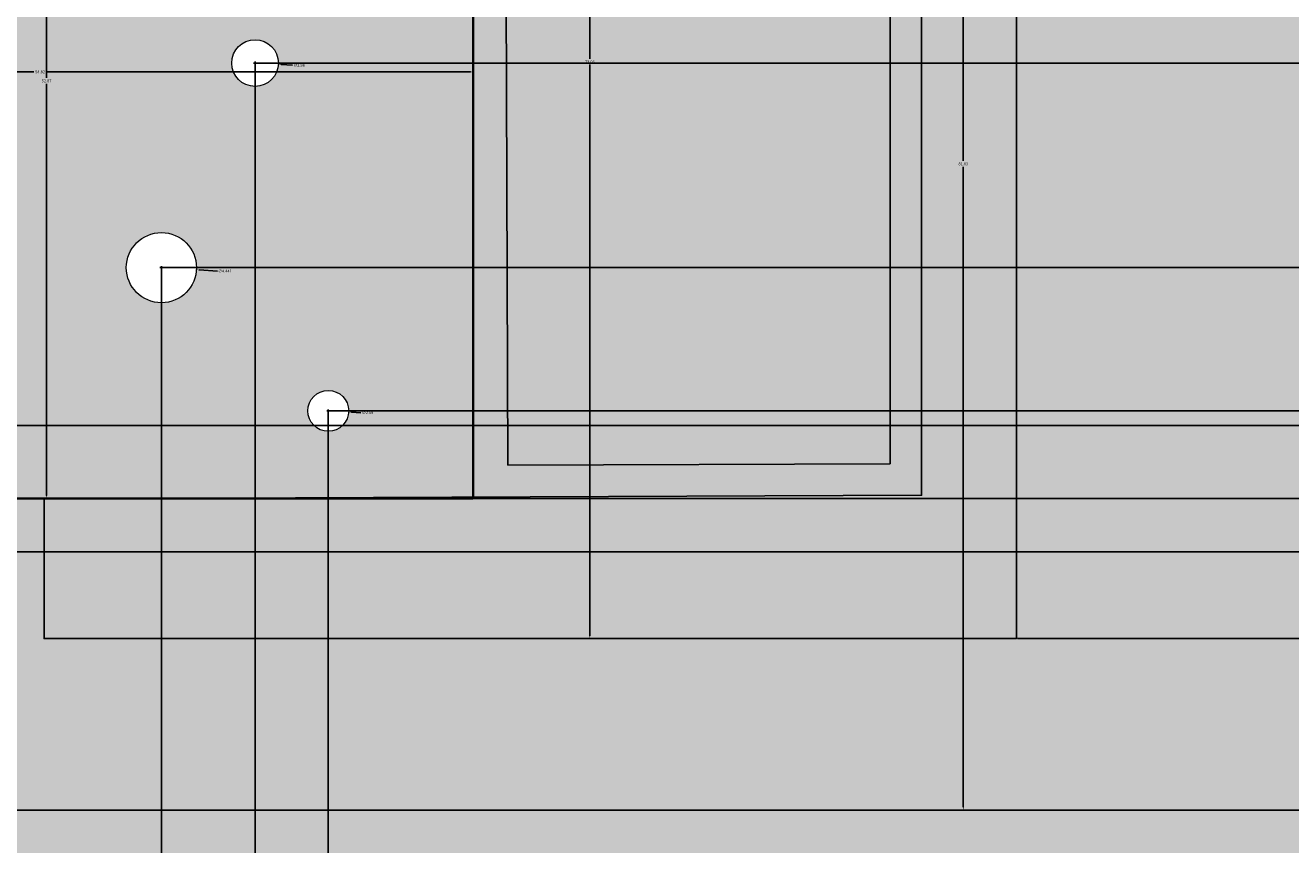
# Model space of a CAD drawing. Units: inches. Extents: x 73 to 607, y 92 to 651.
# Tile 4 of 18: x 368 to 448, y 173 to 224. Entities that reach past the tile are written whole.
import ezdxf

# ---------------------------------------------------------------- set-up
doc = ezdxf.new("R2010")
doc.units = ezdxf.units.IN
doc.header["$MEASUREMENT"] = 0
for name, color, linetype, lineweight in [('A-ANNO-DIMS', 2, 'Continuous', 18), ('A-ELEV', 7, 'Continuous', 35), ('A-ELEV-PANL', 7, 'Continuous', 18), ('A-ELEV-PATT-BKGD', 252, 'Continuous', 13), ('A-ELEV-PATT-FRAM', 38, 'Continuous', 13), ('A-ELEV-PATT-SHAD', 8, 'Continuous', 13), ('A-ELEV-PATT-WALL', 254, 'Continuous', 13), ('A-ELEV-PATT-WOOD', 32, 'Continuous', 13), ('A-GLAZ', 4, 'Continuous', 25), ('A-GLAZ-PATT', 7, 'Continuous', 13)]:
    doc.layers.add(name, color=color, linetype=linetype, lineweight=lineweight)
doc.styles.get("Standard").update_dxf_attribs({"font": 'arial.ttf'})
doc.dimstyles.get("Standard").update_dxf_attribs({"dimtxt": 0.18, "dimasz": 0.18, "dimexe": 0.18, "dimexo": 0.0625, "dimgap": 0.09, "dimtad": 0, "dimtih": 1, "dimtoh": 1, "dimdec": 4, "dimzin": 0, "dimdsep": 46, "dimtxsty": 'Standard', "dimcen": 0.09, "dimadec": 0, "dimazin": 0, "dimtfac": 1, "dimtdec": 4, "dimtofl": 0, "dimtmove": 0, "dimatfit": 3, "dimfxl": 1, "dimtolj": 1, "dimtzin": 0, "dimarcsym": 0})

# ---------------------------------------------------------------- blocks, each defined once
blk = doc.blocks.new('*D16')
at = {"layer": 'A-ANNO-DIMS', "color": 0, "lineweight": -2, "transparency": 16777216}
for p, q in [((431.133, 185.662), (607.278, 185.662)), ((607.098, 185.482), (607.098, 180.414)), ((607.098, 174.982), (607.098, 180.05)), ((454.767, 174.802), (607.278, 174.802))]:
    blk.add_line(p, q, dxfattribs=at)
at = {"layer": 'A-ANNO-DIMS', "color": 0, "transparency": 16777216}
for points in [[(607.068, 185.482), (607.128, 185.482), (607.098, 185.662)], [(607.068, 174.982), (607.128, 174.982), (607.098, 174.802)]]:
    blk.add_solid(points, dxfattribs=at)
at = {"layer": 'Defpoints', "color": 0, "transparency": 16777216}
for p in [(431.07, 185.662), (607.098, 185.662), (454.705, 174.802)]:
    blk.add_point(p, dxfattribs=at)
at = {"layer": 'A-ANNO-DIMS', "color": 0, "transparency": 16777216, "insert": (607.098, 180.232), "char_height": 0.18, "attachment_point": 5}
blk.add_mtext('\\A1;10.86', dxfattribs=at)
blk = doc.blocks.new('*D17')
at = {"layer": 'A-ANNO-DIMS', "color": 0, "lineweight": -2, "transparency": 16777216}
for p, q in [((580.161, 262.302), (607.278, 262.302)), ((607.098, 262.122), (607.098, 224.164)), ((607.098, 185.842), (607.098, 223.8)), ((431.133, 185.662), (607.278, 185.662))]:
    blk.add_line(p, q, dxfattribs=at)
at = {"layer": 'A-ANNO-DIMS', "color": 0, "transparency": 16777216}
for points in [[(607.068, 262.122), (607.128, 262.122), (607.098, 262.302)], [(607.068, 185.842), (607.128, 185.842), (607.098, 185.662)]]:
    blk.add_solid(points, dxfattribs=at)
at = {"layer": 'Defpoints', "color": 0, "transparency": 16777216}
for p in [(580.098, 262.302), (607.098, 262.302), (431.07, 185.662)]:
    blk.add_point(p, dxfattribs=at)
at = {"layer": 'A-ANNO-DIMS', "color": 0, "transparency": 16777216, "insert": (607.098, 223.982), "char_height": 0.18, "attachment_point": 5}
blk.add_mtext('\\A1;76.64', dxfattribs=at)
blk = doc.blocks.new('*D35')
at = {"layer": 'A-ANNO-DIMS', "color": 0, "lineweight": -2, "transparency": 16777216}
for p, q in [((341.869, 194.608), (341.873, 221.725)), ((342.053, 221.545), (368.892, 221.541)), ((396.516, 221.537), (369.677, 221.541)), ((396.692, 194.599), (396.696, 221.717))]:
    blk.add_line(p, q, dxfattribs=at)
at = {"layer": 'A-ANNO-DIMS', "color": 0, "transparency": 16777216}
for points in [[(342.053, 221.575), (342.053, 221.515), (341.873, 221.545)], [(396.516, 221.567), (396.516, 221.507), (396.696, 221.537)]]:
    blk.add_solid(points, dxfattribs=at)
at = {"layer": 'Defpoints', "color": 0, "transparency": 16777216}
for p in [(396.696, 221.537), (341.869, 194.545), (396.692, 194.537)]:
    blk.add_point(p, dxfattribs=at)
at = {"layer": 'A-ANNO-DIMS', "color": 0, "transparency": 16777216, "insert": (369.285, 221.541), "char_height": 0.18, "attachment_point": 5}
blk.add_mtext('\\A1;54.82', dxfattribs=at)
blk = doc.blocks.new('*D36')
at = {"layer": 'A-ANNO-DIMS', "color": 0, "lineweight": -2, "transparency": 16777216}
for p, q in [((396.63, 247.405), (369.512, 247.405)), ((369.692, 247.225), (369.692, 221.153)), ((369.692, 194.717), (369.692, 220.789)), ((396.63, 194.537), (369.512, 194.537))]:
    blk.add_line(p, q, dxfattribs=at)
at = {"layer": 'A-ANNO-DIMS', "color": 0, "transparency": 16777216}
for points in [[(369.662, 247.225), (369.722, 247.225), (369.692, 247.405)], [(369.662, 194.717), (369.722, 194.717), (369.692, 194.537)]]:
    blk.add_solid(points, dxfattribs=at)
at = {"layer": 'Defpoints', "color": 0, "transparency": 16777216}
for p in [(369.692, 247.405), (396.692, 247.405), (396.692, 194.537)]:
    blk.add_point(p, dxfattribs=at)
at = {"layer": 'A-ANNO-DIMS', "color": 0, "transparency": 16777216, "insert": (369.692, 220.971), "char_height": 0.18, "attachment_point": 5}
blk.add_mtext('\\A1;52.87', dxfattribs=at)
blk = doc.blocks.new('*D38')
at = {"layer": 'A-ANNO-DIMS', "color": 0, "lineweight": -2, "transparency": 16777216}
for p, q in [((431.008, 258.691), (403.89, 258.691)), ((404.07, 258.511), (404.07, 222.359)), ((404.07, 185.842), (404.07, 221.995)), ((431.008, 185.662), (403.89, 185.662))]:
    blk.add_line(p, q, dxfattribs=at)
at = {"layer": 'A-ANNO-DIMS', "color": 0, "transparency": 16777216}
for points in [[(404.04, 258.511), (404.1, 258.511), (404.07, 258.691)], [(404.04, 185.842), (404.1, 185.842), (404.07, 185.662)]]:
    blk.add_solid(points, dxfattribs=at)
at = {"layer": 'Defpoints', "color": 0, "transparency": 16777216}
for p in [(404.07, 258.691), (431.07, 258.691), (431.07, 185.662)]:
    blk.add_point(p, dxfattribs=at)
at = {"layer": 'A-ANNO-DIMS', "color": 0, "transparency": 16777216, "insert": (404.07, 222.177), "char_height": 0.18, "attachment_point": 5}
blk.add_mtext('\\A1;73.03', dxfattribs=at)
blk = doc.blocks.new('*D40')
at = {"layer": 'A-ANNO-DIMS', "color": 0, "lineweight": -2, "transparency": 16777216}
for p, q in [((454.642, 256.632), (427.525, 256.632)), ((427.705, 256.452), (427.705, 215.899)), ((427.705, 174.982), (427.705, 215.535)), ((454.642, 174.802), (427.525, 174.802))]:
    blk.add_line(p, q, dxfattribs=at)
at = {"layer": 'A-ANNO-DIMS', "color": 0, "transparency": 16777216}
for points in [[(427.675, 256.452), (427.735, 256.452), (427.705, 256.632)], [(427.675, 174.982), (427.735, 174.982), (427.705, 174.802)]]:
    blk.add_solid(points, dxfattribs=at)
at = {"layer": 'Defpoints', "color": 0, "transparency": 16777216}
for p in [(427.705, 256.632), (454.705, 256.632), (454.705, 174.802)]:
    blk.add_point(p, dxfattribs=at)
at = {"layer": 'A-ANNO-DIMS', "color": 0, "transparency": 16777216, "insert": (427.705, 215.717), "char_height": 0.18, "attachment_point": 5}
blk.add_mtext('\\A1;81.83', dxfattribs=at)
blk = doc.blocks.new('*D88')
at = {"layer": 'A-ANNO-DIMS', "color": 0, "lineweight": -2, "transparency": 16777216}
for p, q in [((376.96, 209.081), (376.96, 116.024)), ((363.256, 199.089), (363.256, 116.024)), ((363.436, 116.204), (369.654, 116.204)), ((376.78, 116.204), (370.563, 116.204))]:
    blk.add_line(p, q, dxfattribs=at)
at = {"layer": 'A-ANNO-DIMS', "color": 0, "transparency": 16777216}
for points in [[(363.436, 116.234), (363.436, 116.174), (363.256, 116.204)], [(376.78, 116.234), (376.78, 116.174), (376.96, 116.204)]]:
    blk.add_solid(points, dxfattribs=at)
at = {"layer": 'Defpoints', "color": 0, "transparency": 16777216}
for p in [(376.96, 209.143), (363.256, 199.151), (376.96, 116.204)]:
    blk.add_point(p, dxfattribs=at)
at = {"layer": 'A-ANNO-DIMS', "color": 0, "transparency": 16777216, "insert": (370.108, 116.204), "char_height": 0.18, "attachment_point": 5}
blk.add_mtext('\\A1;13.704', dxfattribs=at)
blk = doc.blocks.new('*D89')
at = {"layer": 'A-ANNO-DIMS', "color": 0, "lineweight": -2, "transparency": 16777216}
for p, q in [((382.886, 222.034), (382.886, 116.024)), ((376.96, 209.081), (376.96, 116.024)), ((377.14, 116.204), (379.53, 116.204)), ((382.706, 116.204), (380.317, 116.204))]:
    blk.add_line(p, q, dxfattribs=at)
at = {"layer": 'A-ANNO-DIMS', "color": 0, "transparency": 16777216}
for points in [[(377.14, 116.234), (377.14, 116.174), (376.96, 116.204)], [(382.706, 116.234), (382.706, 116.174), (382.886, 116.204)]]:
    blk.add_solid(points, dxfattribs=at)
at = {"layer": 'Defpoints', "color": 0, "transparency": 16777216}
for p in [(382.886, 222.096), (376.96, 209.143), (382.886, 116.204)]:
    blk.add_point(p, dxfattribs=at)
at = {"layer": 'A-ANNO-DIMS', "color": 0, "transparency": 16777216, "insert": (379.923, 116.204), "char_height": 0.18, "attachment_point": 5}
blk.add_mtext('\\A1;5.926', dxfattribs=at)
blk = doc.blocks.new('*D90')
at = {"layer": 'A-ANNO-DIMS', "color": 0, "lineweight": -2, "transparency": 16777216}
for p, q in [((382.886, 222.034), (382.886, 116.024)), ((387.516, 200.014), (387.516, 116.024)), ((383.066, 116.204), (384.874, 116.204)), ((387.336, 116.204), (385.529, 116.204))]:
    blk.add_line(p, q, dxfattribs=at)
at = {"layer": 'A-ANNO-DIMS', "color": 0, "transparency": 16777216}
for points in [[(383.066, 116.234), (383.066, 116.174), (382.886, 116.204)], [(387.336, 116.234), (387.336, 116.174), (387.516, 116.204)]]:
    blk.add_solid(points, dxfattribs=at)
at = {"layer": 'Defpoints', "color": 0, "transparency": 16777216}
for p in [(382.886, 222.096), (387.516, 200.076), (387.516, 116.204)]:
    blk.add_point(p, dxfattribs=at)
at = {"layer": 'A-ANNO-DIMS', "color": 0, "transparency": 16777216, "insert": (385.201, 116.204), "char_height": 0.18, "attachment_point": 5}
blk.add_mtext('\\A1;4.63', dxfattribs=at)
blk = doc.blocks.new('*D94')
at = {"layer": 'A-ANNO-DIMS', "color": 0, "lineweight": -2, "transparency": 16777216}
for p, q in [((377.023, 209.143), (607.278, 209.143)), ((607.098, 208.963), (607.098, 204.329)), ((607.098, 199.331), (607.098, 203.965)), ((363.319, 199.151), (607.278, 199.151))]:
    blk.add_line(p, q, dxfattribs=at)
at = {"layer": 'A-ANNO-DIMS', "color": 0, "transparency": 16777216}
for points in [[(607.068, 208.963), (607.128, 208.963), (607.098, 209.143)], [(607.068, 199.331), (607.128, 199.331), (607.098, 199.151)]]:
    blk.add_solid(points, dxfattribs=at)
at = {"layer": 'Defpoints', "color": 0, "transparency": 16777216}
for p in [(376.96, 209.143), (363.256, 199.151), (607.098, 199.151)]:
    blk.add_point(p, dxfattribs=at)
at = {"layer": 'A-ANNO-DIMS', "color": 0, "transparency": 16777216, "insert": (607.098, 204.147), "char_height": 0.18, "attachment_point": 5}
blk.add_mtext('\\A1;9.992', dxfattribs=at)
blk = doc.blocks.new('*D95')
at = {"layer": 'A-ANNO-DIMS', "color": 0, "lineweight": -2, "transparency": 16777216}
for p, q in [((363.874, 225.982), (607.278, 225.982)), ((607.098, 225.802), (607.098, 212.749)), ((607.098, 199.331), (607.098, 212.385)), ((363.319, 199.151), (607.278, 199.151))]:
    blk.add_line(p, q, dxfattribs=at)
at = {"layer": 'A-ANNO-DIMS', "color": 0, "transparency": 16777216}
for points in [[(607.068, 225.802), (607.128, 225.802), (607.098, 225.982)], [(607.068, 199.331), (607.128, 199.331), (607.098, 199.151)]]:
    blk.add_solid(points, dxfattribs=at)
at = {"layer": 'Defpoints', "color": 0, "transparency": 16777216}
for p in [(363.812, 225.982), (607.098, 225.982), (363.256, 199.151)]:
    blk.add_point(p, dxfattribs=at)
at = {"layer": 'A-ANNO-DIMS', "color": 0, "transparency": 16777216, "insert": (607.098, 212.567), "char_height": 0.18, "attachment_point": 5}
blk.add_mtext('\\A1;26.83', dxfattribs=at)
blk = doc.blocks.new('*D97')
at = {"layer": 'A-ANNO-DIMS', "color": 0, "lineweight": -2, "transparency": 16777216}
for p, q in [((387.579, 200.076), (607.278, 200.076)), ((607.098, 199.896), (607.098, 197.488)), ((607.098, 194.717), (607.098, 197.125)), ((396.755, 194.537), (607.278, 194.537))]:
    blk.add_line(p, q, dxfattribs=at)
at = {"layer": 'A-ANNO-DIMS', "color": 0, "transparency": 16777216}
for points in [[(607.068, 199.896), (607.128, 199.896), (607.098, 200.076)], [(607.068, 194.717), (607.128, 194.717), (607.098, 194.537)]]:
    blk.add_solid(points, dxfattribs=at)
at = {"layer": 'Defpoints', "color": 0, "transparency": 16777216}
for p in [(387.516, 200.076), (607.098, 200.076), (396.692, 194.537)]:
    blk.add_point(p, dxfattribs=at)
at = {"layer": 'A-ANNO-DIMS', "color": 0, "transparency": 16777216, "insert": (607.098, 197.306), "char_height": 0.18, "attachment_point": 5}
blk.add_mtext('\\A1;5.54', dxfattribs=at)
blk = doc.blocks.new('*D98')
at = {"layer": 'A-ANNO-DIMS', "color": 0, "lineweight": -2, "transparency": 16777216}
for p, q in [((377.023, 209.143), (607.278, 209.143)), ((607.098, 208.963), (607.098, 204.792)), ((607.098, 200.256), (607.098, 204.428)), ((387.579, 200.076), (607.278, 200.076))]:
    blk.add_line(p, q, dxfattribs=at)
at = {"layer": 'A-ANNO-DIMS', "color": 0, "transparency": 16777216}
for points in [[(607.068, 208.963), (607.128, 208.963), (607.098, 209.143)], [(607.068, 200.256), (607.128, 200.256), (607.098, 200.076)]]:
    blk.add_solid(points, dxfattribs=at)
at = {"layer": 'Defpoints', "color": 0, "transparency": 16777216}
for p in [(376.96, 209.143), (607.098, 209.143), (387.516, 200.076)]:
    blk.add_point(p, dxfattribs=at)
at = {"layer": 'A-ANNO-DIMS', "color": 0, "transparency": 16777216, "insert": (607.098, 204.61), "char_height": 0.18, "attachment_point": 5}
blk.add_mtext('\\A1;9.067', dxfattribs=at)
blk = doc.blocks.new('*D99')
at = {"layer": 'A-ANNO-DIMS', "color": 0, "lineweight": -2, "transparency": 16777216}
for p, q in [((373.319, 231.348), (607.278, 231.348)), ((607.098, 231.168), (607.098, 220.428)), ((607.098, 209.323), (607.098, 220.064)), ((377.023, 209.143), (607.278, 209.143))]:
    blk.add_line(p, q, dxfattribs=at)
at = {"layer": 'A-ANNO-DIMS', "color": 0, "transparency": 16777216}
for points in [[(607.068, 231.168), (607.128, 231.168), (607.098, 231.348)], [(607.068, 209.323), (607.128, 209.323), (607.098, 209.143)]]:
    blk.add_solid(points, dxfattribs=at)
at = {"layer": 'Defpoints', "color": 0, "transparency": 16777216}
for p in [(373.257, 231.348), (607.098, 231.348), (376.96, 209.143)]:
    blk.add_point(p, dxfattribs=at)
at = {"layer": 'A-ANNO-DIMS', "color": 0, "transparency": 16777216, "insert": (607.098, 220.246), "char_height": 0.18, "attachment_point": 5}
blk.add_mtext('\\A1;22.205', dxfattribs=at)
blk = doc.blocks.new('*D100')
at = {"layer": 'A-ANNO-DIMS', "color": 0, "lineweight": -2, "transparency": 16777216}
for p, q in [((382.949, 222.096), (607.278, 222.096)), ((607.098, 221.916), (607.098, 211.268)), ((607.098, 200.256), (607.098, 210.904)), ((387.579, 200.076), (607.278, 200.076))]:
    blk.add_line(p, q, dxfattribs=at)
at = {"layer": 'A-ANNO-DIMS', "color": 0, "transparency": 16777216}
for points in [[(607.068, 221.916), (607.128, 221.916), (607.098, 222.096)], [(607.068, 200.256), (607.128, 200.256), (607.098, 200.076)]]:
    blk.add_solid(points, dxfattribs=at)
at = {"layer": 'Defpoints', "color": 0, "transparency": 16777216}
for p in [(382.886, 222.096), (607.098, 222.096), (387.516, 200.076)]:
    blk.add_point(p, dxfattribs=at)
at = {"layer": 'A-ANNO-DIMS', "color": 0, "transparency": 16777216, "insert": (607.098, 211.086), "char_height": 0.18, "attachment_point": 5}
blk.add_mtext('\\A1;22.02', dxfattribs=at)
blk = doc.blocks.new('*D101')
at = {"layer": 'A-ANNO-DIMS', "color": 0, "lineweight": -2, "transparency": 16777216}
for p, q in [((382.393, 240.97), (607.278, 240.97)), ((607.098, 240.79), (607.098, 231.715)), ((607.098, 222.276), (607.098, 231.351)), ((382.949, 222.096), (607.278, 222.096))]:
    blk.add_line(p, q, dxfattribs=at)
at = {"layer": 'A-ANNO-DIMS', "color": 0, "transparency": 16777216}
for points in [[(607.068, 240.79), (607.128, 240.79), (607.098, 240.97)], [(607.068, 222.276), (607.128, 222.276), (607.098, 222.096)]]:
    blk.add_solid(points, dxfattribs=at)
at = {"layer": 'Defpoints', "color": 0, "transparency": 16777216}
for p in [(382.331, 240.97), (607.098, 240.97), (382.886, 222.096)]:
    blk.add_point(p, dxfattribs=at)
at = {"layer": 'A-ANNO-DIMS', "color": 0, "transparency": 16777216, "insert": (607.098, 231.533), "char_height": 0.18, "attachment_point": 5}
blk.add_mtext('\\A1;18.874', dxfattribs=at)
blk = doc.blocks.new('*D119')
at = {"layer": 'A-ANNO-DIMS', "color": 0, "lineweight": -2, "transparency": 16777216}
for p, q in [((469.817, 191.142), (72.918, 191.142)), ((73.098, 190.962), (73.098, 183.154)), ((73.098, 174.982), (73.098, 182.79)), ((454.642, 174.802), (72.918, 174.802))]:
    blk.add_line(p, q, dxfattribs=at)
at = {"layer": 'A-ANNO-DIMS', "color": 0, "transparency": 16777216}
for points in [[(73.068, 190.962), (73.128, 190.962), (73.098, 191.142)], [(73.068, 174.982), (73.128, 174.982), (73.098, 174.802)]]:
    blk.add_solid(points, dxfattribs=at)
at = {"layer": 'Defpoints', "color": 0, "transparency": 16777216}
for p in [(73.098, 191.142), (469.879, 191.142), (454.705, 174.802)]:
    blk.add_point(p, dxfattribs=at)
at = {"layer": 'A-ANNO-DIMS', "color": 0, "transparency": 16777216, "insert": (73.098, 182.972), "char_height": 0.18, "attachment_point": 5}
blk.add_mtext('\\A1;16.34', dxfattribs=at)
blk = doc.blocks.new('*D149')
at = {"layer": 'A-ANNO-DIMS', "color": 0, "lineweight": -2, "transparency": 16777216}
for p, q in [((382.796, 222.096), (382.976, 222.096)), ((382.886, 222.006), (382.886, 222.186)), ((385.251, 221.954), (384.544, 221.997))]:
    blk.add_line(p, q, dxfattribs=at)
at = {"layer": 'A-ANNO-DIMS', "color": 0, "transparency": 16777216}
blk.add_solid([(384.546, 222.027), (384.542, 221.967), (384.364, 222.008)], dxfattribs=at)
at = {"layer": 'Defpoints', "color": 0, "transparency": 16777216}
for p in [(381.409, 222.185), (384.364, 222.008)]:
    blk.add_point(p, dxfattribs=at)
at = {"layer": 'A-ANNO-DIMS', "color": 0, "transparency": 16777216, "insert": (385.672, 221.954), "char_height": 0.18, "attachment_point": 5}
blk.add_mtext('\\A1;∅2.96', dxfattribs=at)
blk = doc.blocks.new('*D151')
at = {"layer": 'A-ANNO-DIMS', "color": 0, "lineweight": -2, "transparency": 16777216}
for p, q in [((376.87, 209.143), (377.05, 209.143)), ((376.96, 209.053), (376.96, 209.233)), ((380.507, 208.928), (379.356, 208.998))]:
    blk.add_line(p, q, dxfattribs=at)
at = {"layer": 'A-ANNO-DIMS', "color": 0, "transparency": 16777216}
blk.add_solid([(379.358, 209.028), (379.355, 208.968), (379.177, 209.009)], dxfattribs=at)
at = {"layer": 'Defpoints', "color": 0, "transparency": 16777216}
for p in [(374.744, 209.278), (379.177, 209.009)]:
    blk.add_point(p, dxfattribs=at)
at = {"layer": 'A-ANNO-DIMS', "color": 0, "transparency": 16777216, "insert": (380.981, 208.928), "char_height": 0.18, "attachment_point": 5}
blk.add_mtext('\\A1;∅4.441', dxfattribs=at)
blk = doc.blocks.new('*D153')
at = {"layer": 'A-ANNO-DIMS', "color": 0, "lineweight": -2, "transparency": 16777216}
for p, q in [((387.426, 200.076), (387.606, 200.076)), ((387.516, 199.986), (387.516, 200.166)), ((389.585, 199.961), (388.989, 199.994))]:
    blk.add_line(p, q, dxfattribs=at)
at = {"layer": 'A-ANNO-DIMS', "color": 0, "transparency": 16777216}
blk.add_solid([(388.991, 200.024), (388.987, 199.965), (388.809, 200.004)], dxfattribs=at)
at = {"layer": 'Defpoints', "color": 0, "transparency": 16777216}
for p in [(386.223, 200.148), (388.809, 200.004)]:
    blk.add_point(p, dxfattribs=at)
at = {"layer": 'A-ANNO-DIMS', "color": 0, "transparency": 16777216, "insert": (390.007, 199.961), "char_height": 0.18, "attachment_point": 5}
blk.add_mtext('\\A1;∅2.59', dxfattribs=at)

msp = doc.modelspace()

# ---------------------------------------------------------------- hatches: boundary and pattern name
at = {"layer": 'A-ELEV-PATT-BKGD'}
h = msp.add_hatch(color=256, dxfattribs=at)
h.dxf.hatch_style = 1
h.paths.add_polyline_path([(321.3008, 479.2042), (312.3008, 479.2042), (312.3008, 478.7576), (312.3008, 412.636), (321.3008, 412.636)])
h.paths.add_polyline_path([(312.3008, 504.7576), (256.4726, 504.7576), (256.4726, 503.4576), (312.3008, 503.4576)], flags=17)
h.paths.add_polyline_path([(321.3008, 543.1576), (321.3008, 552.1576), (320.3257, 552.1576), (312.3008, 552.1576), (256.4726, 552.1576), (256.4726, 543.1576), (312.3008, 543.1576), (312.3008, 479.2042), (321.3008, 479.2042)])
h.paths.add_polyline_path([(451.5214, 412.636), (256.4726, 412.636), (256.4726, 403.636), (442.5214, 403.636), (442.5214, 320.2042), (206.1343, 320.2042), (206.1343, 320.9135), (206.1343, 403.636), (256.4726, 403.636), (256.4726, 412.636), (201.6343, 412.636), (201.6343, 320.9135), (201.6343, 320.2042), (201.6343, 311.2042), (256.4726, 311.2042), (451.5214, 311.2042)])
h.paths.add_polyline_path([(431.07, 258.6914), (369.5339, 258.6914), (369.5339, 247.4054), (396.692, 247.4054), (425.07, 247.4054), (425.07, 194.7312), (396.692, 194.6197), (396.692, 194.5366), (369.5339, 194.5366), (369.5339, 185.6619), (431.07, 185.6619)])
h.paths.add_polyline_path([(580.0983, 262.3024), (451.5214, 262.3024), (451.5214, 143.2042), (580.0983, 143.2042)])
h.paths.add_polyline_path([(454.7049, 174.802), (454.7049, 256.6321), (577.9249, 256.6321), (577.9249, 174.802)], flags=16)
h.paths.add_polyline_path([(465.9716, 191.1416, -1), (473.7874, 191.1416, -1)], flags=0)
h.paths.add_polyline_path([(490.5373, 181.6586, -1), (494.9999, 181.6586, -1)], flags=0)
h.paths.add_polyline_path([(476.2996, 209.8287, -1), (500.5844, 209.8287, -1)], flags=0)
h.paths.add_polyline_path([(505.3326, 194.7675, -1), (512.5843, 194.7675, -1)], flags=0)
h.paths.add_polyline_path([(520.9613, 186.679, -1), (526.544, 186.679, -1)], flags=0)
h.paths.add_polyline_path([(466.8103, 225.7267, -1), (470.1573, 225.7267, -1)], flags=0)
h.paths.add_polyline_path([(527.1059, 203.6926, -1), (536.0311, 203.6926, -1)], flags=0)
h.paths.add_polyline_path([(504.775, 232.6995, -1), (513.7002, 232.6995, -1)], flags=0)
h.paths.add_polyline_path([(546.9241, 183.611, -1), (554.7336, 183.611, -1)], flags=0)
h.paths.add_polyline_path([(459.5544, 243.856, -1), (466.8061, 243.856, -1)], flags=0)
h.paths.add_polyline_path([(476.3045, 246.924, -1), (488.5767, 246.924, -1)], flags=0)
h.paths.add_polyline_path([(529.9044, 226.8424, -1), (556.68, 226.8424, -1)], flags=0)
h.paths.add_polyline_path([(554.1814, 203.9716, -1), (561.4331, 203.9716, -1)], flags=0)
h.paths.add_polyline_path([(567.8561, 193.3729, -1), (570.6475, 193.3729, -1)], flags=0)
h.paths.add_polyline_path([(522.3584, 250.271, -1), (525.7053, 250.271, -1)], flags=0)
h.paths.add_polyline_path([(561.9965, 245.2506, -1), (567.5748, 245.2506, -1)], flags=0)
h.paths.add_polyline_path([(347.8686, 194.5366), (341.8686, 194.5366), (341.8686, 194.5452), (314.0144, 194.5452), (314.0144, 188.5452), (347.8686, 188.5452)])
h.paths.add_polyline_path([(347.8686, 253.4054), (314.0144, 253.4054), (314.0144, 247.4054), (341.8686, 247.4054), (347.8686, 247.4054)])
h.paths.add_polyline_path([(304.3559, 253.4054), (298.3559, 253.4054), (298.3559, 188.5452), (304.3559, 188.5452)])
h.paths.add_polyline_path([(450.6603, 552.1576), (369.9727, 552.1576), (369.9727, 479.2042), (374.4727, 479.2042), (374.4727, 547.6576), (446.1603, 547.6576), (446.1603, 479.2042), (450.6603, 479.2042)])
h.paths.add_polyline_path([(374.4727, 479.2042), (369.9727, 479.2042), (369.9727, 465.0632), (374.4727, 465.0632)])
h.paths.add_polyline_path([(450.6603, 479.2042), (446.1603, 479.2042), (446.1603, 465.0632), (450.6603, 465.0632)])
h.paths.add_polyline_path([(256.4726, 281.6039), (109.0983, 281.6039), (100.0983, 281.6039), (100.0983, 167.2042), (100.0983, 143.2042), (109.0983, 143.2042), (109.0983, 167.2042), (109.0983, 272.6039), (256.4726, 272.6039)])
at = {"layer": 'A-ELEV-PATT-FRAM'}
h = msp.add_hatch(color=256, dxfattribs=at)
h.dxf.hatch_style = 1
h.paths.add_polyline_path([(433.025, 403.636), (409.515, 403.636), (409.515, 342.1009), (411.515, 342.1009), (411.515, 401.636), (431.025, 401.636), (431.025, 342.1009), (433.025, 342.1009)])
h.paths.add_polyline_path([(433.025, 341.1009), (431.025, 341.1009), (431.025, 340.0025), (411.515, 340.0025), (411.515, 341.1009), (409.515, 341.1009), (409.515, 338.0025), (433.025, 338.0025)])
h.paths.add_polyline_path([(425.07, 247.4054), (396.692, 247.4054), (396.692, 194.6197), (425.07, 194.7312)])
h.paths.add_polyline_path([(423.07, 245.4054), (423.07, 196.7234), (398.8836, 196.6284), (398.692, 245.4054)], flags=16)
h.paths.add_polyline_path([(341.8686, 247.4054), (314.0144, 247.4054), (314.0144, 245.4054), (339.8686, 245.4054), (339.8686, 196.5452), (314.0144, 196.5452), (314.0144, 194.5452), (341.8686, 194.5452)])
h.paths.add_polyline_path([(372.3213, 383.1812), (350.3213, 383.1812), (350.3213, 342.1009), (372.3213, 342.1009)], flags=16)
h.paths.add_polyline_path([(376.3213, 389.1812), (346.3213, 389.1812), (346.3213, 342.1009), (350.3213, 342.1009), (350.3213, 383.1812), (372.3213, 383.1812), (372.3213, 342.1009), (376.3213, 342.1009)], flags=17)
h.paths.add_polyline_path([(375.3213, 362.2042, -1), (373.3213, 362.2042, -1)], flags=16)
h.paths.add_polyline_path([(379.3213, 392.2042), (343.3213, 392.2042), (343.3213, 342.1009), (346.3213, 342.1009), (346.3213, 389.1812), (376.3213, 389.1812), (376.3213, 342.1009), (379.3213, 342.1009)])
h.paths.add_polyline_path([(350.3213, 341.1009), (346.3213, 341.1009), (346.3213, 338.0025), (350.3213, 338.0025)])
h.paths.add_polyline_path([(346.3213, 341.1009), (343.3213, 341.1009), (343.3213, 338.0025), (346.3213, 338.0025)])
h.paths.add_polyline_path([(346.3213, 337.0025), (343.3213, 337.0025), (343.3213, 332.9397), (346.3213, 332.9397)])
h.paths.add_polyline_path([(350.3213, 337.0025), (346.3213, 337.0025), (346.3213, 332.9397), (350.3213, 332.9397)])
h.paths.add_polyline_path([(350.3213, 331.9397), (346.3213, 331.9397), (346.3213, 320.2042), (376.3213, 320.2042), (376.3213, 331.9397), (372.3213, 331.9397), (372.3213, 326.2042), (350.3213, 326.2042)])
h.paths.add_polyline_path([(372.3213, 337.0025), (350.3213, 337.0025), (350.3213, 332.9397), (372.3213, 332.9397)])
h.paths.add_polyline_path([(372.3213, 341.1009), (350.3213, 341.1009), (350.3213, 338.0025), (372.3213, 338.0025)])
h.paths.add_polyline_path([(376.3213, 341.1009), (372.3213, 341.1009), (372.3213, 338.0025), (376.3213, 338.0025)])
h.paths.add_polyline_path([(376.3213, 337.0025), (372.3213, 337.0025), (372.3213, 332.9397), (376.3213, 332.9397)])
h.paths.add_polyline_path([(379.3213, 341.1009), (376.3213, 341.1009), (376.3213, 338.0025), (379.3213, 338.0025)])
h.paths.add_polyline_path([(379.3213, 337.0025), (376.3213, 337.0025), (376.3213, 332.9397), (379.3213, 332.9397)])
h.paths.add_polyline_path([(379.3213, 331.9397), (376.3213, 331.9397), (376.3213, 320.2042), (379.3213, 320.2042)])
h.paths.add_polyline_path([(372.3213, 331.9397), (350.3213, 331.9397), (350.3213, 326.2042), (372.3213, 326.2042)], flags=17)
h.paths.add_polyline_path([(346.3213, 331.9397), (343.3213, 331.9397), (343.3213, 320.2042), (346.3213, 320.2042)])
at = {"layer": 'A-ELEV-PATT-SHAD'}
h = msp.add_hatch(color=256, dxfattribs=at)
h.dxf.hatch_style = 1
h.paths.add_polyline_path([(451.5214, 412.636), (256.4726, 412.636), (256.4726, 403.636), (442.5214, 403.636), (442.5214, 320.2042), (206.1343, 320.2042), (206.1343, 320.9135), (206.1343, 403.636), (256.4726, 403.636), (256.4726, 412.636), (201.6343, 412.636), (201.6343, 320.9135), (201.6343, 320.2042), (201.6343, 311.2042), (256.4726, 311.2042), (451.5214, 311.2042)])
h.paths.add_polyline_path([(580.0983, 262.3024), (451.5214, 262.3024), (451.5214, 143.2042), (580.0983, 143.2042)])
h.paths.add_polyline_path([(454.7049, 174.802), (454.7049, 256.6321), (577.9249, 256.6321), (577.9249, 174.802)], flags=16)
h.paths.add_polyline_path([(465.9716, 191.1416, -1), (473.7874, 191.1416, -1)], flags=0)
h.paths.add_polyline_path([(490.5373, 181.6586, -1), (494.9999, 181.6586, -1)], flags=0)
h.paths.add_polyline_path([(476.2996, 209.8287, -1), (500.5844, 209.8287, -1)], flags=0)
h.paths.add_polyline_path([(505.3326, 194.7675, -1), (512.5843, 194.7675, -1)], flags=0)
h.paths.add_polyline_path([(520.9613, 186.679, -1), (526.544, 186.679, -1)], flags=0)
h.paths.add_polyline_path([(466.8103, 225.7267, -1), (470.1573, 225.7267, -1)], flags=0)
h.paths.add_polyline_path([(527.1059, 203.6926, -1), (536.0311, 203.6926, -1)], flags=0)
h.paths.add_polyline_path([(459.5544, 243.856, -1), (466.8061, 243.856, -1)], flags=0)
h.paths.add_polyline_path([(504.775, 232.6995, -1), (513.7002, 232.6995, -1)], flags=0)
h.paths.add_polyline_path([(476.3045, 246.924, -1), (488.5767, 246.924, -1)], flags=0)
h.paths.add_polyline_path([(546.9241, 183.611, -1), (554.7336, 183.611, -1)], flags=0)
h.paths.add_polyline_path([(529.9044, 226.8424, -1), (556.68, 226.8424, -1)], flags=0)
h.paths.add_polyline_path([(554.1814, 203.9716, -1), (561.4331, 203.9716, -1)], flags=0)
h.paths.add_polyline_path([(522.3584, 250.271, -1), (525.7053, 250.271, -1)], flags=0)
h.paths.add_polyline_path([(567.8561, 193.3729, -1), (570.6475, 193.3729, -1)], flags=0)
h.paths.add_polyline_path([(561.9965, 245.2506, -1), (567.5748, 245.2506, -1)], flags=0)
h.paths.add_polyline_path([(431.07, 258.6914), (369.5339, 258.6914), (369.5339, 247.4054), (396.692, 247.4054), (425.07, 247.4054), (425.07, 194.7312), (396.692, 194.6197), (396.692, 194.5366), (369.5339, 194.5366), (369.5339, 185.6619), (431.07, 185.6619)])
h.paths.add_polyline_path([(347.8686, 253.4054), (314.0144, 253.4054), (314.0144, 247.4054), (341.8686, 247.4054), (347.8686, 247.4054)])
h.paths.add_polyline_path([(304.3559, 253.4054), (298.3559, 253.4054), (298.3559, 188.5452), (304.3559, 188.5452)])
h.paths.add_polyline_path([(347.8686, 194.5366), (341.8686, 194.5366), (341.8686, 194.5452), (314.0144, 194.5452), (314.0144, 188.5452), (347.8686, 188.5452)])
at = {"layer": 'A-ELEV-PATT-WALL'}
h = msp.add_hatch(color=256, dxfattribs=at)
h.dxf.hatch_style = 1
h.paths.add_polyline_path([(509.9692, 483.857), (450.6603, 483.857), (450.6603, 465.0632), (446.1603, 465.0632), (446.1603, 484.2142), (374.4727, 484.2142), (374.4727, 465.0632), (369.9727, 465.0632), (369.9727, 484.2142), (321.3008, 484.2142), (321.3008, 412.636), (451.5214, 412.636), (451.5214, 311.2042), (314.0144, 311.2042), (314.0144, 253.4054), (347.8686, 253.4054), (347.8686, 247.4054), (369.5339, 247.4054), (369.5339, 258.6914), (431.07, 258.6914), (431.07, 185.6619), (369.5339, 185.6619), (369.5339, 194.5366), (347.8686, 194.5366), (347.8686, 188.5452), (314.0144, 188.5452), (314.0144, 143.2042), (451.5214, 143.2042), (451.5214, 262.3024), (580.0983, 262.3024), (580.0983, 311.2042), (509.9692, 311.2042)])
h.paths.add_polyline_path([(304.3559, 311.2042), (256.4726, 311.2042), (256.4726, 167.2042), (256.4726, 143.2042), (304.3559, 143.2042), (304.3559, 188.5452), (298.3559, 188.5452), (298.3559, 253.4054), (304.3559, 253.4054)])
at = {"layer": 'A-ELEV-PATT-WOOD'}
h = msp.add_hatch(color=256, dxfattribs=at)
h.dxf.hatch_style = 1
h.paths.add_polyline_path([(396.692, 247.4054), (341.8686, 247.4054), (341.8686, 194.5366), (375.5339, 194.5366), (396.692, 194.6197)])
h.paths.add_polyline_path([(390.6634, 232.4585, -1), (388.443, 232.4585, -1)], flags=16)
h.paths.add_polyline_path([(384.3667, 222.0962, -1), (381.4061, 222.0962, -1)], flags=16)
h.paths.add_polyline_path([(380.8505, 240.9703, -1), (383.8112, 240.9703, -1)], flags=16)
h.paths.add_polyline_path([(371.9613, 231.3482, -1), (374.5519, 231.3482, -1)], flags=16)
h.paths.add_polyline_path([(363.0718, 225.982, -1), (364.5521, 225.982, -1)], flags=16)
h.paths.add_polyline_path([(379.1808, 209.1433, -1), (374.7399, 209.1433, -1)], flags=16)
h.paths.add_polyline_path([(357.8883, 238.9349, -1), (363.8096, 238.9349, -1)], flags=16)
h.paths.add_polyline_path([(362.6961, 213.0292, -1), (350.8535, 213.0292, -1)], flags=16)
h.paths.add_polyline_path([(388.8114, 200.0764, -1), (386.2208, 200.0764, -1)], flags=16)
h.paths.add_polyline_path([(352.6976, 226.5372, -1), (345.296, 226.5372, -1)], flags=16)
h.paths.add_polyline_path([(347.3301, 237.4546, -1), (350.6635, 237.4546, -1)], flags=16)
h.paths.add_polyline_path([(363.9971, 199.1512, -1), (362.5156, 199.1512, -1)], flags=16)
at = {"layer": 'A-GLAZ-PATT'}
h = msp.add_hatch(color=256, dxfattribs=at)
h.dxf.hatch_style = 1
h.set_gradient(color1=(0, 0, 255))
h.paths.add_polyline_path([(423.07, 245.4054), (398.692, 245.4054), (398.8836, 196.6284), (423.07, 196.7234)])

# ---------------------------------------------------------------- linework, layer by layer
at = {"layer": 'A-ELEV'}
msp.add_lwpolyline([(341.8686, 247.4054), (396.692, 247.4054), (396.692, 194.5366), (341.8686, 194.5366)], close=True, dxfattribs=at)
at = {"layer": 'A-ELEV-PANL'}
for centre, radius in [((382.8864, 222.0962), 1.4803), ((376.9603, 209.1433), 2.2205), ((387.5161, 200.0764), 1.2953)]:
    msp.add_circle(centre, radius, dxfattribs=at)
at = {"layer": 'A-GLAZ'}
msp.add_line((398.692, 245.4054), (398.8836, 196.6284), dxfattribs=at)
for points in [[(369.5339, 247.4054), (369.5339, 258.6914), (431.07, 258.6914), (431.07, 185.6619), (369.5339, 185.6619), (369.5339, 194.5366)], [(375.5339, 247.4054), (425.07, 247.4054), (425.07, 194.7312), (375.5339, 194.5366)], [(398.692, 245.4054), (423.07, 245.4054), (423.07, 196.7234), (398.8836, 196.6284)]]:
    msp.add_lwpolyline(points, dxfattribs=at)

# ---------------------------------------------------------------- dimensions: what is measured, and where the dimension line sits
at = {"layer": 'A-ANNO-DIMS'}
for base, p1, p2, angle, override, picture, middle in [((607.0983, 262.3024), (431.07, 185.6619), (580.0983, 262.3024), 90, {"dimdec": 2, "dimlfac": 1, "dimrnd": 0, "dimzin": 0, "dimdsep": 46, "dimlunit": 2}, '*D17', (607.0983, 223.9821)), ((404.07, 258.6914), (431.07, 185.6619), (431.07, 258.6914), 90, {"dimdec": 2, "dimlfac": 1, "dimrnd": 0, "dimzin": 0, "dimdsep": 46, "dimlunit": 2}, '*D38', (404.07, 222.1767)), ((427.7049, 256.6321), (454.7049, 174.802), (454.7049, 256.6321), 90, {"dimdec": 2, "dimlfac": 1, "dimrnd": 0, "dimzin": 0, "dimdsep": 46, "dimlunit": 2}, '*D40', (427.7049, 215.7171)), ((369.692, 247.4054), (396.692, 194.5366), (396.692, 247.4054), 90, {"dimdec": 2, "dimlfac": 1, "dimrnd": 0, "dimzin": 0, "dimdsep": 46, "dimlunit": 2}, '*D36', (369.692, 220.971)), ((607.0983, 240.9703), (382.8864, 222.0962), (382.3308, 240.9703), 90, {"dimdec": 3, "dimlfac": 1, "dimrnd": 0, "dimzin": 0, "dimdsep": 46, "dimlunit": 2}, '*D101', (607.0983, 231.5333)), ((607.0983, 231.3482), (376.9603, 209.1433), (373.2566, 231.3482), 90, {"dimdec": 3, "dimlfac": 1, "dimrnd": 0, "dimzin": 0, "dimdsep": 46, "dimlunit": 2}, '*D99', (607.0983, 220.2458)), ((607.0983, 225.982), (363.2564, 199.1512), (363.8119, 225.982), 90, {"dimdec": 2, "dimlfac": 1, "dimrnd": 0, "dimzin": 0, "dimdsep": 46, "dimlunit": 2}, '*D95', (607.0983, 212.5666)), ((607.0983, 222.0962), (387.5161, 200.0764), (382.8864, 222.0962), 90, {"dimdec": 2, "dimlfac": 1, "dimrnd": 0, "dimzin": 0, "dimdsep": 46, "dimlunit": 2}, '*D100', (607.0983, 211.0863)), ((396.6962, 221.5366), (341.8686, 194.5452), (396.692, 194.5366), 359.991065, {"dimdec": 2, "dimlfac": 1, "dimrnd": 0, "dimzin": 0, "dimdsep": 46, "dimlunit": 2}, '*D35', (369.2845, 221.5409)), ((607.0983, 199.1512), (376.9603, 209.1433), (363.2564, 199.1512), 90, {"dimdec": 3, "dimlfac": 1, "dimrnd": 0, "dimzin": 0, "dimdsep": 46, "dimlunit": 2}, '*D94', (607.0983, 204.1472)), ((607.0983, 209.1433), (387.5161, 200.0764), (376.9603, 209.1433), 90, {"dimdec": 3, "dimlfac": 1, "dimrnd": 0, "dimzin": 0, "dimdsep": 46, "dimlunit": 2}, '*D98', (607.0983, 204.6098)), ((607.0983, 200.0764), (396.692, 194.5366), (387.5161, 200.0764), 90, {"dimdec": 2, "dimlfac": 1, "dimrnd": 0, "dimzin": 0, "dimdsep": 46, "dimlunit": 2}, '*D97', (607.0983, 197.3065)), ((73.0983, 191.1416), (454.7049, 174.802), (469.8795, 191.1416), 90, {"dimdec": 2, "dimlfac": 1, "dimrnd": 0, "dimzin": 0, "dimdsep": 46, "dimlunit": 2}, '*D119', (73.0983, 182.9718)), ((607.0983, 185.6619), (454.7049, 174.802), (431.07, 185.6619), 90, {"dimdec": 2, "dimlfac": 1, "dimrnd": 0, "dimzin": 0, "dimdsep": 46, "dimlunit": 2}, '*D16', (607.0983, 180.232))]:
    dim = msp.add_linear_dim(base=base, p1=p1, p2=p2, angle=angle, dimstyle='Standard', override=override, dxfattribs=at)
    dim.commit()
    dim.dimension.update_dxf_attribs({"geometry": picture, "text_midpoint": middle})
for base, p1, p2, override, picture, middle in [((382.8864, 116.2042), (376.9603, 209.1433), (382.8864, 222.0962), {"dimdec": 3, "dimlfac": 1, "dimrnd": 0, "dimzin": 0, "dimdsep": 46, "dimlunit": 2}, '*D89', (379.9234, 116.2042)), ((387.5161, 116.2042), (382.8864, 222.0962), (387.5161, 200.0764), {"dimdec": 2, "dimlfac": 1, "dimrnd": 0, "dimzin": 0, "dimdsep": 46, "dimlunit": 2}, '*D90', (385.2013, 116.2042)), ((376.9603, 116.2042), (363.2564, 199.1512), (376.9603, 209.1433), {"dimdec": 3, "dimlfac": 1, "dimrnd": 0, "dimzin": 0, "dimdsep": 46, "dimlunit": 2}, '*D88', (370.1084, 116.2042))]:
    dim = msp.add_linear_dim(base=base, p1=p1, p2=p2, dimstyle='Standard', override=override, dxfattribs=at)
    dim.commit()
    dim.dimension.update_dxf_attribs({"geometry": picture, "text_midpoint": middle})
for p1, p2, override, picture, middle in [((381.4087, 222.1848), (384.3641, 222.0076), {"dimdec": 2, "dimlfac": 1, "dimrnd": 0, "dimzin": 0, "dimdsep": 46, "dimlunit": 2}, '*D149', (385.2507, 221.9544)), ((374.7439, 209.278), (379.1768, 209.0087), {"dimdec": 3, "dimlfac": 1, "dimrnd": 0, "dimzin": 0, "dimdsep": 46, "dimlunit": 2}, '*D151', (380.5066, 208.9279)), ((386.2228, 200.1482), (388.8094, 200.0045), {"dimdec": 2, "dimlfac": 1, "dimrnd": 0, "dimzin": 0, "dimdsep": 46, "dimlunit": 2}, '*D153', (389.5854, 199.9614))]:
    dim = msp.add_diameter_dim_2p(p1=p1, p2=p2, dimstyle='Standard', override=override, dxfattribs=at)
    dim.commit()
    dim.dimension.update_dxf_attribs({"geometry": picture, "text_midpoint": middle, "dimtype": 163})

doc.saveas('drawing.dxf')
